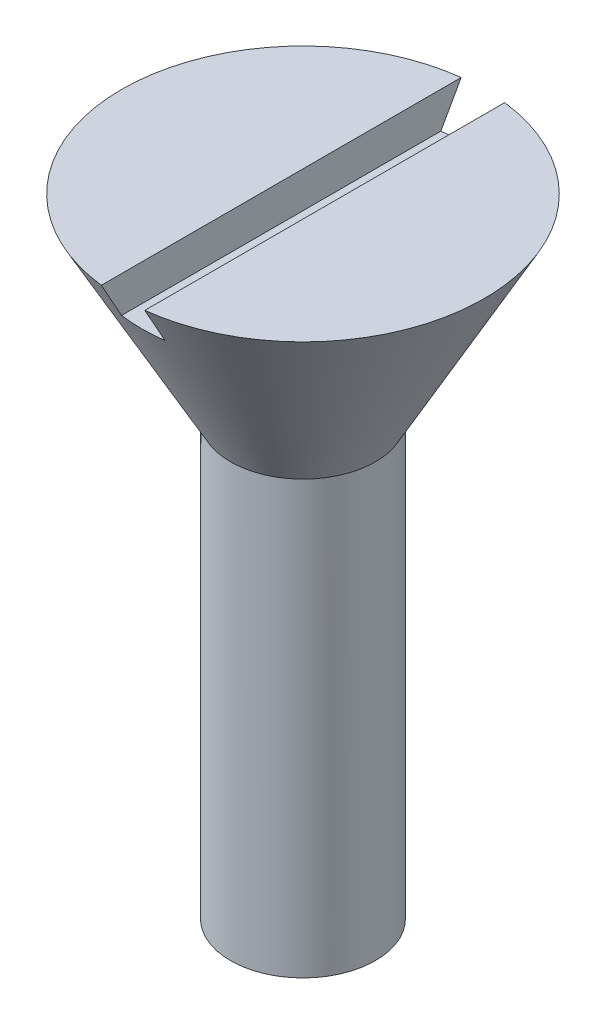
SolidWorks part; units mm, degrees
material "Plain Carbon Steel"
ref_plane "Front Plane" through (0, 0, 0) normal (0, 0, 1) x (1, 0, 0)
ref_plane "Top Plane" through (0, 0, 0) normal (0, 1, 0) x (1, 0, 0)
ref_plane "Right Plane" through (0, 0, 0) normal (1, 0, 0) x (0, 0, -1)
sketch "Screw Half Profile Sketch" plane through (0, 0, 0) normal (0, 0, 1) x (1, 0, 0)
  line L0 (0, 0) -> (5, 0)
  line L1 (5, 0) -> (5, 50)
  line L2 (5, 50) -> (15, 68)
  line L3 (15, 68) -> (0, 68)
  line L4 (0, 68) -> (0, 0)
  dimension "D1" = 5
  dimension "D2" = 68
  dimension "D3" = 15
  dimension "D4" = 50
revolve "Screw Body Revolve" add sketch "Screw Half Profile Sketch" angle 360 about L4
sketch "Head Slot Sketch" plane through (0, 0, 0) normal (0, 0, 1) x (1, 0, 0)
  line L0 (15, 68) -> (-15, 68) construction
  line L1 (-1.5, 68) -> (1.5, 68)
  line L2 (-1.5, 68) -> (-1.5, 61)
  line L3 (-1.5, 61) -> (1.5, 61)
  line L4 (1.5, 68) -> (1.5, 61)
  line L5 (0, 0) -> (0, 120.3338) construction
  dimension "D1" = 3
  dimension "D2" = 7
extrude "Head Slot Cut" cut sketch "Head Slot Sketch" against normal through all both and the other way through all
sketch "Trim Cut 1 Sketch" plane through (0, 0, 0) normal (0, 0, 1) x (1, 0, 0)
  line L0 (-1.5, 68) -> (-15, 68) construction
  line L1 (-15, 68) -> (15.2811, 68)
  line L2 (-15, 68) -> (-15, 63.5017)
  line L3 (-15, 63.5017) -> (15.2811, 63.5017)
  line L4 (15.2811, 68) -> (15.2811, 63.5017)
  dimension "D1" = 30.2811
  dimension "D2" = 4.4983
  dimension "D3" = 15
extrude "Trim Cut 1" cut sketch "Trim Cut 1 Sketch" against normal through all both and the other way through all
sketch "Trim Cut 2 Sketch" plane through (0, 0, 0) normal (0, 0, 1) x (1, 0, 0)
  line L1 (-18.1656, 20.2041) -> (10.9187, 20.2041)
  line L2 (-18.1656, 20.2041) -> (-18.1656, 0)
  line L3 (-18.1656, 0) -> (10.9187, 0)
  line L4 (10.9187, 20.2041) -> (10.9187, 0)
  dimension "D1" = 29.0843
  dimension "D2" = 20.2041
  dimension "D3" = 18.1656
extrude "Trim Cut 2" cut sketch "Trim Cut 2 Sketch" along normal through all both and the other way through all
